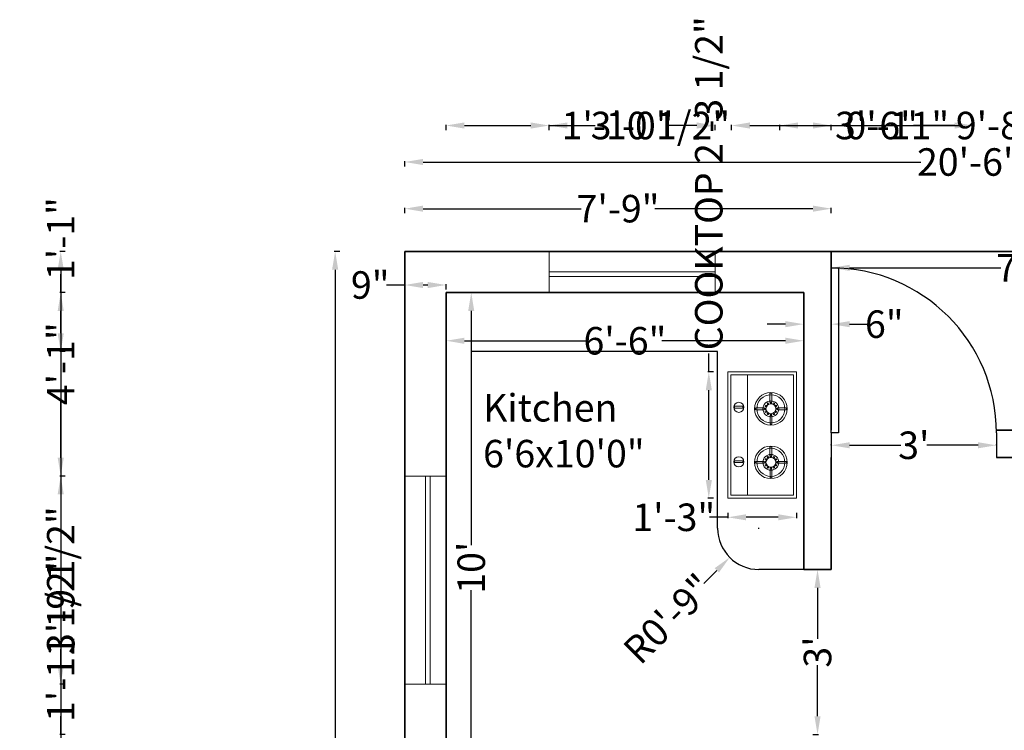
# Model space of a CAD drawing. Units: inches. Extents: x -81 to 380, y -521 to 79.
# Tile 3 of 5: x -81 to 134, y -76 to 79. Entities that reach past the tile are written whole.
import ezdxf

# ---------------------------------------------------------------- set-up
doc = ezdxf.new("R2010")
doc.units = ezdxf.units.IN
doc.header["$MEASUREMENT"] = 0
for name, color, linetype, lineweight in [('A-ANNO-DIMS', 2, 'Continuous', 18), ('A-AREA-IDEN', 5, 'Continuous', 25), ('A-EQPM', 8, 'Continuous', 18), ('A-FLOR-CASE', 249, 'Continuous', 25), ('A-GLAZ', 4, 'Continuous', 18), ('A-WALL', 249, 'Continuous', 35), ('door', 34, 'Continuous', 25)]:
    doc.layers.add(name, color=color, linetype=linetype, lineweight=lineweight)
doc.styles.get("Standard").update_dxf_attribs({"font": 'arial.ttf'})
doc.dimstyles.get("Standard").update_dxf_attribs({"dimtxt": 6, "dimasz": 4, "dimexe": 0.18, "dimexo": 0.0625, "dimgap": 0.09, "dimtad": 0, "dimdec": 0, "dimzin": 0, "dimdsep": 46, "dimlunit": 3, "dimtxsty": 'Standard', "dimcen": 0.09, "dimclrd": 6, "dimclre": 6, "dimclrt": 2, "dimadec": 0, "dimazin": 0, "dimtfac": 1, "dimtdec": 0, "dimtofl": 0, "dimtmove": 0, "dimatfit": 3, "dimfxl": 1, "dimfxlon": 1, "dimtolj": 1, "dimtzin": 0, "dimarcsym": 0})

# ---------------------------------------------------------------- blocks, each defined once
blk = doc.blocks.new('*U2')
for p, q in [((0, 0), (0, -6)), ((40, 0), (40, -6))]:
    blk.add_line(p, q)
blk.add_lwpolyline([(0, 0), (0, 40), (1.75, 40), (1.75, 0)], close=True)
blk.add_arc((0, 0), 40, 0, 90)
blk = doc.blocks.new('*D5')
at = {"layer": 'A-ANNO-DIMS', "color": 0, "lineweight": -2, "transparency": 16777216}
for p, q in [((3.31, 46.97), (3.31, 48.15)), ((7.31, 47.97), (115.86, 47.97)), ((245.31, 47.97), (136.76, 47.97)), ((249.31, 46.97), (249.31, 48.15))]:
    blk.add_line(p, q, dxfattribs=at)
at = {"layer": 'A-ANNO-DIMS', "color": 0, "transparency": 16777216}
for points in [[(7.31, 48.64), (7.31, 47.3), (3.31, 47.97)], [(245.31, 48.64), (245.31, 47.3), (249.31, 47.97)]]:
    blk.add_solid(points, dxfattribs=at)
at = {"layer": 'Defpoints', "color": 0, "transparency": 16777216}
for p in [(249.31, 47.97), (3.31, 28.48), (249.31, 28.48)]:
    blk.add_point(p, dxfattribs=at)
at = {"layer": 'A-ANNO-DIMS', "color": 0, "transparency": 16777216, "insert": (126.31, 47.97), "char_height": 6, "attachment_point": 5}
blk.add_mtext('\\A1;20\'-6"', dxfattribs=at)
blk = doc.blocks.new('*D6')
at = {"layer": 'A-ANNO-DIMS', "color": 0, "lineweight": -2, "transparency": 16777216}
for p, q in [((3.31, 21.14), (-0.69, 21.14)), ((3.31, 20.14), (3.31, 21.32)), ((8.31, 21.14), (7.31, 21.14)), ((12.31, 20.14), (12.31, 21.32))]:
    blk.add_line(p, q, dxfattribs=at)
at = {"layer": 'A-ANNO-DIMS', "color": 0, "transparency": 16777216}
for points in [[(7.31, 21.81), (7.31, 20.47), (3.31, 21.14)], [(8.31, 21.81), (8.31, 20.47), (12.31, 21.14)]]:
    blk.add_solid(points, dxfattribs=at)
at = {"layer": 'Defpoints', "color": 0, "transparency": 16777216}
for p in [(3.31, 21.14), (3.31, 19.48), (12.31, 19.48)]:
    blk.add_point(p, dxfattribs=at)
at = {"layer": 'A-ANNO-DIMS', "color": 0, "transparency": 16777216, "insert": (-4.23, 21.14), "char_height": 6, "attachment_point": 5}
blk.add_mtext('\\A1;9"', dxfattribs=at)
blk = doc.blocks.new('*D7')
at = {"layer": 'A-ANNO-DIMS', "color": 0, "lineweight": -2, "transparency": 16777216}
for p, q in [((90.31, 12.9), (90.31, 12.42)), ((96.31, 12.9), (96.31, 12.42)), ((86.31, 12.6), (82.31, 12.6)), ((100.31, 12.6), (104.31, 12.6))]:
    blk.add_line(p, q, dxfattribs=at)
at = {"layer": 'A-ANNO-DIMS', "color": 0, "transparency": 16777216}
for points in [[(86.31, 13.26), (86.31, 11.93), (90.31, 12.6)], [(100.31, 13.26), (100.31, 11.93), (96.31, 12.6)]]:
    blk.add_solid(points, dxfattribs=at)
at = {"layer": 'Defpoints', "color": 0, "transparency": 16777216}
for p in [(90.31, 12.96), (96.31, 12.96), (96.31, 12.6)]:
    blk.add_point(p, dxfattribs=at)
at = {"layer": 'A-ANNO-DIMS', "color": 0, "transparency": 16777216, "insert": (107.87, 12.6), "char_height": 6, "attachment_point": 5}
blk.add_mtext('\\A1;6"', dxfattribs=at)
blk = doc.blocks.new('*D8')
at = {"layer": 'A-ANNO-DIMS', "color": 0, "lineweight": -2, "transparency": 16777216}
for p, q in [((-10.88, 28.48), (-12.06, 28.48)), ((-11.88, 24.48), (-11.88, -110.29)), ((-11.88, -255.52), (-11.88, -120.75)), ((-10.88, -259.52), (-12.06, -259.52))]:
    blk.add_line(p, q, dxfattribs=at)
at = {"layer": 'A-ANNO-DIMS', "color": 0, "transparency": 16777216}
for points in [[(-12.55, 24.48), (-11.21, 24.48), (-11.88, 28.48)], [(-12.55, -255.52), (-11.21, -255.52), (-11.88, -259.52)]]:
    blk.add_solid(points, dxfattribs=at)
at = {"layer": 'Defpoints', "color": 0, "transparency": 16777216}
for p in [(3.31, 28.48), (-11.88, -259.52), (3.31, -259.52)]:
    blk.add_point(p, dxfattribs=at)
at = {"layer": 'A-ANNO-DIMS', "color": 0, "transparency": 16777216, "insert": (-11.88, -115.52), "char_height": 6, "attachment_point": 5, "rotation": 90}
blk.add_mtext("\\A1;24'", dxfattribs=at)
blk = doc.blocks.new('*D12')
at = {"layer": 'A-ANNO-DIMS', "color": 0, "lineweight": -2, "transparency": 16777216}
for p, q in [((3.31, 36.79), (3.31, 37.97)), ((7.31, 37.79), (41.77, 37.79)), ((92.31, 37.79), (57.85, 37.79)), ((96.31, 36.79), (96.31, 37.97))]:
    blk.add_line(p, q, dxfattribs=at)
at = {"layer": 'A-ANNO-DIMS', "color": 0, "transparency": 16777216}
for points in [[(7.31, 38.46), (7.31, 37.12), (3.31, 37.79)], [(92.31, 38.46), (92.31, 37.12), (96.31, 37.79)]]:
    blk.add_solid(points, dxfattribs=at)
at = {"layer": 'Defpoints', "color": 0, "transparency": 16777216}
for p in [(96.31, 37.79), (3.31, 28.48), (96.31, 28.48)]:
    blk.add_point(p, dxfattribs=at)
at = {"layer": 'A-ANNO-DIMS', "color": 0, "transparency": 16777216, "insert": (49.81, 37.79), "char_height": 6, "attachment_point": 5}
blk.add_mtext('\\A1;7\'-9"', dxfattribs=at)
blk = doc.blocks.new('*D13')
at = {"layer": 'A-ANNO-DIMS', "color": 0, "lineweight": -2, "transparency": 16777216}
for p, q in [((18.8, 19.48), (17.62, 19.48)), ((17.8, 15.48), (17.8, -35.62)), ((17.8, -96.52), (17.8, -45.42)), ((18.8, -100.52), (17.62, -100.52))]:
    blk.add_line(p, q, dxfattribs=at)
at = {"layer": 'A-ANNO-DIMS', "color": 0, "transparency": 16777216}
for points in [[(17.13, 15.48), (18.46, 15.48), (17.8, 19.48)], [(17.13, -96.52), (18.46, -96.52), (17.8, -100.52)]]:
    blk.add_solid(points, dxfattribs=at)
at = {"layer": 'Defpoints', "color": 0, "transparency": 16777216}
for p in [(17.8, 19.48), (28.81, 19.48), (28.81, -100.52)]:
    blk.add_point(p, dxfattribs=at)
at = {"layer": 'A-ANNO-DIMS', "color": 0, "transparency": 16777216, "insert": (17.8, -40.52), "char_height": 6, "attachment_point": 5, "rotation": 90}
blk.add_mtext("\\A1;10'", dxfattribs=at)
blk = doc.blocks.new('*D14')
at = {"layer": 'A-ANNO-DIMS', "color": 0, "lineweight": -2, "transparency": 16777216}
for p, q in [((12.31, 8.08), (12.31, 9.16)), ((16.31, 8.98), (43.23, 8.98)), ((86.31, 8.98), (59.39, 8.98)), ((90.31, 8.98), (90.31, 9.16))]:
    blk.add_line(p, q, dxfattribs=at)
at = {"layer": 'A-ANNO-DIMS', "color": 0, "transparency": 16777216}
for points in [[(16.31, 9.65), (16.31, 8.31), (12.31, 8.98)], [(86.31, 9.65), (86.31, 8.31), (90.31, 8.98)]]:
    blk.add_solid(points, dxfattribs=at)
at = {"layer": 'Defpoints', "color": 0, "transparency": 16777216}
for p in [(90.31, 8.98), (90.31, 8.98), (12.31, 8.01)]:
    blk.add_point(p, dxfattribs=at)
at = {"layer": 'A-ANNO-DIMS', "color": 0, "transparency": 16777216, "insert": (51.31, 8.98), "char_height": 6, "attachment_point": 5}
blk.add_mtext('\\A1;6\'-6"', dxfattribs=at)
blk = doc.blocks.new('*D15')
at = {"layer": 'A-ANNO-DIMS', "color": 0, "lineweight": -2, "transparency": 16777216}
for p, q in [((96.31, 24.88), (96.31, 25.06)), ((100.31, 24.88), (133.27, 24.88)), ((182.31, 24.88), (149.35, 24.88)), ((186.31, 24.88), (186.31, 25.06))]:
    blk.add_line(p, q, dxfattribs=at)
at = {"layer": 'A-ANNO-DIMS', "color": 0, "transparency": 16777216}
for points in [[(100.31, 25.55), (100.31, 24.21), (96.31, 24.88)], [(182.31, 25.55), (182.31, 24.21), (186.31, 24.88)]]:
    blk.add_solid(points, dxfattribs=at)
at = {"layer": 'Defpoints', "color": 0, "transparency": 16777216}
for p in [(96.31, 24.88), (186.31, 24.88), (186.31, 24.88)]:
    blk.add_point(p, dxfattribs=at)
at = {"layer": 'A-ANNO-DIMS', "color": 0, "transparency": 16777216, "insert": (141.31, 24.88), "char_height": 6, "attachment_point": 5}
blk.add_mtext('\\A1;7\'-6"', dxfattribs=at)
blk = doc.blocks.new('*D27')
at = {"layer": 'A-ANNO-DIMS', "color": 0, "lineweight": -2, "transparency": 16777216}
for p, q in [((96.31, -13.82), (96.31, -13.64)), ((100.31, -13.82), (111.46, -13.82)), ((128.31, -13.82), (117.16, -13.82)), ((132.31, -13.82), (132.31, -13.64))]:
    blk.add_line(p, q, dxfattribs=at)
at = {"layer": 'A-ANNO-DIMS', "color": 0, "transparency": 16777216}
for points in [[(100.31, -13.15), (100.31, -14.49), (96.31, -13.82)], [(128.31, -13.15), (128.31, -14.49), (132.31, -13.82)]]:
    blk.add_solid(points, dxfattribs=at)
at = {"layer": 'Defpoints', "color": 0, "transparency": 16777216}
for p in [(96.31, -13.82), (132.31, -13.82), (132.31, -13.82)]:
    blk.add_point(p, dxfattribs=at)
at = {"layer": 'A-ANNO-DIMS', "color": 0, "transparency": 16777216, "insert": (114.31, -13.82), "char_height": 6, "attachment_point": 5}
blk.add_mtext("\\A1;3'", dxfattribs=at)
blk = doc.blocks.new('*D28')
at = {"layer": 'A-ANNO-DIMS', "color": 0, "lineweight": -2, "transparency": 16777216}
for p, q in [((92.31, -40.92), (93.49, -40.92)), ((93.31, -44.92), (93.31, -56.07)), ((93.31, -72.92), (93.31, -61.76)), ((92.31, -76.92), (93.49, -76.92))]:
    blk.add_line(p, q, dxfattribs=at)
at = {"layer": 'A-ANNO-DIMS', "color": 0, "transparency": 16777216}
for points in [[(92.64, -44.92), (93.98, -44.92), (93.31, -40.92)], [(92.64, -72.92), (93.98, -72.92), (93.31, -76.92)]]:
    blk.add_solid(points, dxfattribs=at)
at = {"layer": 'Defpoints', "color": 0, "transparency": 16777216}
for p in [(90.31, -40.92), (93.31, -40.92), (90.31, -76.92)]:
    blk.add_point(p, dxfattribs=at)
at = {"layer": 'A-ANNO-DIMS', "color": 0, "transparency": 16777216, "insert": (93.31, -58.92), "char_height": 6, "attachment_point": 5, "rotation": 90}
blk.add_mtext("\\A1;3'", dxfattribs=at)
blk = doc.blocks.new('A$C06E242FC')
for p, q in [((0, 455.6), (0.5, 456.1)), ((0, 455.6), (0, 0.5)), ((838.9, 456.1), (0.5, 456.1)), ((20, 435.6), (20.5, 436.1)), ((20, 435.6), (20, 20.5)), ((818.9, 436.1), (20.5, 436.1)), ((237.3, 411.5), (237.3, 356.2)), ((248.9, 411.5), (237.3, 411.5)), ((248.9, 356.2), (248.9, 411.5)), ((599.3, 411.5), (610.9, 411.5)), ((599.3, 411.5), (599.3, 356.2)), ((610.9, 356.2), (610.9, 411.5)), ((819.4, 435.6), (818.9, 436.1)), ((819.4, 20.5), (819.4, 435.6)), ((838.9, 456.1), (839.4, 455.6)), ((839.4, 0.5), (839.4, 455.6)), ((237.3, 356.2), (248.9, 356.2)), ((599.3, 356.2), (610.9, 356.2)), ((20, 324.4), (819.4, 324.4)), ((232.7, 272.7), (232.7, 214)), ((244.9, 272.7), (232.7, 272.7)), ((244.9, 214), (244.9, 272.7)), ((588.1, 272.7), (588.1, 214)), ((600.3, 272.7), (588.1, 272.7)), ((600.3, 214), (600.3, 272.7)), ((232.7, 214), (244.9, 214)), ((588.1, 214), (600.3, 214)), ((136.3, 176), (136.3, 163.8)), ((194.9, 176), (136.3, 176)), ((136.3, 163.8), (194.9, 163.8)), ((194.9, 163.8), (194.9, 176)), ((282.9, 176.3), (282.9, 164.1)), ((341.6, 176.3), (282.9, 176.3)), ((282.9, 164.1), (341.6, 164.1)), ((341.6, 164.1), (341.6, 176.3)), ((550.3, 176), (491.7, 176)), ((491.7, 176), (491.7, 163.8)), ((491.7, 163.8), (550.3, 163.8)), ((550.3, 163.8), (550.3, 176)), ((638.3, 176.3), (638.3, 164.1)), ((697, 176.3), (638.3, 176.3)), ((638.3, 164.1), (697, 164.1)), ((697, 164.1), (697, 176.3)), ((245.2, 126.1), (233, 126.1)), ((233, 126.1), (233, 67.4)), ((233, 67.4), (245.2, 67.4)), ((245.2, 67.4), (245.2, 126.1)), ((600.6, 126.1), (588.3, 126.1)), ((588.3, 126.1), (588.3, 67.4)), ((588.3, 67.4), (600.6, 67.4)), ((600.6, 67.4), (600.6, 126.1)), ((0, 0.5), (0.5, 0)), ((20, 20.5), (20.5, 20)), ((20.5, 20), (818.9, 20)), ((818.9, 20), (819.4, 20.5)), ((838.9, 0), (839.4, 0.5)), ((0.5, 0), (838.9, 0))]:
    blk.add_line(p, q)
for centre, radius in [((242, 382.9), 33.3), ((604.1, 382.9), 33.3), ((238.9, 170.1), 108.3), ((238.9, 170.1), 93.3), ((594.3, 170.1), 108.3), ((594.3, 170.1), 93.3), ((238.9, 170.1), 52.6), ((238.9, 170.1), 32.6), ((219.5, 203.7), 4.84), ((238.9, 208.9), 4.84), ((258.4, 203.7), 4.84), ((594.3, 170.1), 52.6), ((594.3, 170.1), 32.6), ((574.9, 203.7), 4.84), ((594.3, 208.9), 4.84), ((613.7, 203.7), 4.84), ((200.1, 170.1), 4.84), ((205.3, 189.5), 4.84), ((205.3, 150.6), 4.84), ((219.5, 136.4), 4.84), ((238.9, 131.2), 4.84), ((258.4, 136.4), 4.84), ((272.6, 189.5), 4.84), ((272.6, 150.6), 4.84), ((277.8, 170.1), 4.84), ((555.5, 170.1), 4.84), ((560.7, 189.5), 4.84), ((560.7, 150.6), 4.84), ((574.9, 136.4), 4.84), ((594.3, 131.2), 4.84), ((613.7, 136.4), 4.84), ((628, 189.5), 4.84), ((628, 150.6), 4.84), ((633.2, 170.1), 4.84)]:
    blk.add_circle(centre, radius)
blk = doc.blocks.new('*D44')
at = {"layer": 'A-ANNO-DIMS', "color": 6, "lineweight": -2, "transparency": 16777216}
for p, q in [((69.6, 2.19), (69.6, 6.19)), ((70.6, 2.19), (69.42, 2.19)), ((69.6, -21.39), (69.6, -1.81)), ((70.6, -25.39), (69.42, -25.39))]:
    blk.add_line(p, q, dxfattribs=at)
at = {"layer": 'A-ANNO-DIMS', "color": 6, "transparency": 16777216}
for points in [[(68.94, -1.81), (70.27, -1.81), (69.6, 2.19)], [(68.94, -21.39), (70.27, -21.39), (69.6, -25.39)]]:
    blk.add_solid(points, dxfattribs=at)
at = {"layer": 'Defpoints', "color": 0, "transparency": 16777216}
for p in [(69.6, 2.19), (73.74, 2.19), (73.74, -25.39)]:
    blk.add_point(p, dxfattribs=at)
at = {"layer": 'A-ANNO-DIMS', "color": 2, "transparency": 16777216, "insert": (69.6, 43.33), "char_height": 6, "attachment_point": 5, "rotation": 90}
blk.add_mtext('\\A1;COOKTOP 2\'-3 1/2"', dxfattribs=at)
blk = doc.blocks.new('*D45')
at = {"layer": 'A-ANNO-DIMS', "color": 6, "lineweight": -2, "transparency": 16777216}
for p, q in [((73.74, -29.53), (69.74, -29.53)), ((73.74, -28.53), (73.74, -29.71)), ((84.73, -29.53), (77.74, -29.53)), ((88.73, -28.53), (88.73, -29.71))]:
    blk.add_line(p, q, dxfattribs=at)
at = {"layer": 'A-ANNO-DIMS', "color": 6, "transparency": 16777216}
for points in [[(77.74, -28.86), (77.74, -30.2), (73.74, -29.53)], [(84.73, -28.86), (84.73, -30.2), (88.73, -29.53)]]:
    blk.add_solid(points, dxfattribs=at)
at = {"layer": 'Defpoints', "color": 0, "transparency": 16777216}
for p in [(73.74, -25.39), (88.73, -25.39), (73.74, -29.53)]:
    blk.add_point(p, dxfattribs=at)
at = {"layer": 'A-ANNO-DIMS', "color": 2, "transparency": 16777216, "insert": (61.96, -29.53), "char_height": 6, "attachment_point": 5}
blk.add_mtext('\\A1;1\'-3"', dxfattribs=at)
blk = doc.blocks.new('*D46')
at = {"layer": 'A-ANNO-DIMS', "color": 6, "lineweight": -2, "transparency": 16777216}
for p, q in [((74.55, 54.93), (74.55, 56.11)), ((78.55, 55.93), (124.45, 55.93)), ((186.48, 55.93), (140.58, 55.93)), ((190.48, 54.93), (190.48, 56.11))]:
    blk.add_line(p, q, dxfattribs=at)
at = {"layer": 'A-ANNO-DIMS', "color": 6, "transparency": 16777216}
for points in [[(78.55, 56.6), (78.55, 55.26), (74.55, 55.93)], [(186.48, 56.6), (186.48, 55.26), (190.48, 55.93)]]:
    blk.add_solid(points, dxfattribs=at)
at = {"layer": 'Defpoints', "color": 0, "transparency": 16777216}
for p in [(190.48, 55.93), (74.55, -489.67), (190.48, -489.67)]:
    blk.add_point(p, dxfattribs=at)
at = {"layer": 'A-ANNO-DIMS', "color": 2, "transparency": 16777216, "insert": (132.51, 55.93), "char_height": 6, "attachment_point": 5}
blk.add_mtext('\\A1;9\'-8"', dxfattribs=at)
blk = doc.blocks.new('*D48')
at = {"layer": 'A-ANNO-DIMS', "color": 6, "lineweight": -2, "transparency": 16777216}
for p, q in [((-70.72, 28.48), (-71.9, 28.48)), ((-71.72, 24.48), (-71.72, -220.08)), ((-71.72, -485.67), (-71.72, -241.11)), ((-70.72, -489.67), (-71.9, -489.67))]:
    blk.add_line(p, q, dxfattribs=at)
at = {"layer": 'A-ANNO-DIMS', "color": 6, "transparency": 16777216}
for points in [[(-72.39, 24.48), (-71.06, 24.48), (-71.72, 28.48)], [(-72.39, -485.67), (-71.06, -485.67), (-71.72, -489.67)]]:
    blk.add_solid(points, dxfattribs=at)
at = {"layer": 'Defpoints', "color": 0, "transparency": 16777216}
for p in [(3.31, 28.48), (-71.72, -489.67), (74.55, -489.67)]:
    blk.add_point(p, dxfattribs=at)
at = {"layer": 'A-ANNO-DIMS', "color": 2, "transparency": 16777216, "insert": (-71.72, -230.6), "char_height": 6, "attachment_point": 5, "rotation": 90}
blk.add_mtext('\\A1;43\'-2"', dxfattribs=at)
blk = doc.blocks.new('*D50')
at = {"layer": 'A-ANNO-DIMS', "color": 6, "lineweight": -2, "transparency": 16777216}
for p, q in [((85.08, 54.93), (85.08, 56.11)), ((89.08, 55.93), (98.09, 55.93)), ((123.23, 55.93), (114.22, 55.93)), ((127.23, 54.93), (127.23, 56.11))]:
    blk.add_line(p, q, dxfattribs=at)
at = {"layer": 'A-ANNO-DIMS', "color": 6, "transparency": 16777216}
for points in [[(89.08, 56.6), (89.08, 55.26), (85.08, 55.93)], [(123.23, 56.6), (123.23, 55.26), (127.23, 55.93)]]:
    blk.add_solid(points, dxfattribs=at)
at = {"layer": 'Defpoints', "color": 0, "transparency": 16777216}
for p in [(127.23, 55.93), (85.08, -292.11), (127.23, -292.11)]:
    blk.add_point(p, dxfattribs=at)
at = {"layer": 'A-ANNO-DIMS', "color": 2, "transparency": 16777216, "insert": (106.16, 55.93), "char_height": 6, "attachment_point": 5}
blk.add_mtext('\\A1;3\'-6"', dxfattribs=at)
blk = doc.blocks.new('*D53')
at = {"layer": 'A-ANNO-DIMS', "color": 6, "lineweight": -2, "transparency": 16777216}
for p, q in [((85.08, 54.93), (85.08, 56.11)), ((89.08, 55.93), (92.31, 55.93)), ((96.31, 54.93), (96.31, 56.11)), ((96.31, 55.93), (100.31, 55.93))]:
    blk.add_line(p, q, dxfattribs=at)
at = {"layer": 'A-ANNO-DIMS', "color": 6, "transparency": 16777216}
for points in [[(89.08, 56.6), (89.08, 55.26), (85.08, 55.93)], [(92.31, 56.6), (92.31, 55.26), (96.31, 55.93)]]:
    blk.add_solid(points, dxfattribs=at)
at = {"layer": 'Defpoints', "color": 0, "transparency": 16777216}
for p in [(96.31, 55.93), (85.08, -259.52), (96.31, -259.52)]:
    blk.add_point(p, dxfattribs=at)
at = {"layer": 'A-ANNO-DIMS', "color": 2, "transparency": 16777216, "insert": (110.71, 55.93), "char_height": 6, "attachment_point": 5}
blk.add_mtext('\\A1;0\'-11"', dxfattribs=at)
blk = doc.blocks.new('*D54')
at = {"layer": 'A-ANNO-DIMS', "color": 6, "lineweight": -2, "transparency": 16777216}
for p, q in [((370.52, 19.48), (371.7, 19.48)), ((371.52, 15.48), (371.52, 4.34)), ((371.52, -36.92), (371.52, -25.77)), ((370.52, -40.92), (371.7, -40.92))]:
    blk.add_line(p, q, dxfattribs=at)
at = {"layer": 'A-ANNO-DIMS', "color": 6, "transparency": 16777216}
for points in [[(370.86, 15.48), (372.19, 15.48), (371.52, 19.48)], [(370.86, -36.92), (372.19, -36.92), (371.52, -40.92)]]:
    blk.add_solid(points, dxfattribs=at)
at = {"layer": 'Defpoints', "color": 0, "transparency": 16777216}
for p in [(90.31, 19.48), (90.31, -40.92), (371.52, -40.92)]:
    blk.add_point(p, dxfattribs=at)
at = {"layer": 'A-ANNO-DIMS', "color": 2, "transparency": 16777216, "insert": (371.52, -10.72), "char_height": 6, "attachment_point": 5, "rotation": 90}
blk.add_mtext('\\A1;5\'-0 1/2"', dxfattribs=at)
blk = doc.blocks.new('*D55')
at = {"layer": 'A-ANNO-DIMS', "color": 6, "lineweight": -2, "transparency": 16777216}
for p, q in [((67.53, -517.12), (63.53, -517.12)), ((71.53, -516.12), (71.53, -517.3)), ((90.31, -516.12), (90.31, -517.3)), ((94.31, -517.12), (98.31, -517.12))]:
    blk.add_line(p, q, dxfattribs=at)
at = {"layer": 'A-ANNO-DIMS', "color": 6, "transparency": 16777216}
for points in [[(67.53, -516.45), (67.53, -517.79), (71.53, -517.12)], [(94.31, -516.45), (94.31, -517.79), (90.31, -517.12)]]:
    blk.add_solid(points, dxfattribs=at)
at = {"layer": 'Defpoints', "color": 0, "transparency": 16777216}
for p in [(71.53, -31.92), (90.31, -40.92), (90.31, -517.12)]:
    blk.add_point(p, dxfattribs=at)
at = {"layer": 'A-ANNO-DIMS', "color": 2, "transparency": 16777216, "insert": (80.92, -517.12), "char_height": 6, "attachment_point": 5}
blk.add_mtext('\\A1;1\'-7"', dxfattribs=at)
blk = doc.blocks.new('*D56')
at = {"layer": 'A-ANNO-DIMS', "color": 6, "lineweight": -2, "transparency": 16777216}
for p, q in [((-71.72, 19.48), (-71.72, 23.48)), ((-70.72, 19.48), (-71.9, 19.48)), ((-71.72, 10.6), (-71.72, 15.48)), ((-70.72, 6.6), (-71.9, 6.6))]:
    blk.add_line(p, q, dxfattribs=at)
at = {"layer": 'A-ANNO-DIMS', "color": 6, "transparency": 16777216}
for points in [[(-72.39, 15.48), (-71.06, 15.48), (-71.72, 19.48)], [(-72.39, 10.6), (-71.06, 10.6), (-71.72, 6.6)]]:
    blk.add_solid(points, dxfattribs=at)
at = {"layer": 'Defpoints', "color": 0, "transparency": 16777216}
for p in [(-71.72, 19.48), (12.31, 19.48), (17.8, 6.6)]:
    blk.add_point(p, dxfattribs=at)
at = {"layer": 'A-ANNO-DIMS', "color": 2, "transparency": 16777216, "insert": (-71.72, 31.26), "char_height": 6, "attachment_point": 5, "rotation": 90}
blk.add_mtext('\\A1;1\'-1"', dxfattribs=at)
blk = doc.blocks.new('*D57')
at = {"layer": 'A-ANNO-DIMS', "color": 6, "lineweight": -2, "transparency": 16777216}
for p, q in [((-71.72, -76.92), (-71.72, -72.92)), ((-70.72, -76.92), (-71.9, -76.92)), ((-71.72, -96.52), (-71.72, -80.92)), ((-70.72, -100.52), (-71.9, -100.52))]:
    blk.add_line(p, q, dxfattribs=at)
at = {"layer": 'A-ANNO-DIMS', "color": 6, "transparency": 16777216}
for points in [[(-72.39, -80.92), (-71.06, -80.92), (-71.72, -76.92)], [(-72.39, -96.52), (-71.06, -96.52), (-71.72, -100.52)]]:
    blk.add_solid(points, dxfattribs=at)
at = {"layer": 'Defpoints', "color": 0, "transparency": 16777216}
for p in [(-71.72, -76.92), (45.3, -76.92), (45.3, -100.52)]:
    blk.add_point(p, dxfattribs=at)
at = {"layer": 'A-ANNO-DIMS', "color": 2, "transparency": 16777216, "insert": (-71.72, -55.81), "char_height": 6, "attachment_point": 5, "rotation": 90}
blk.add_mtext('\\A1;1\'-11 1/2"', dxfattribs=at)
blk = doc.blocks.new('*D59')
at = {"layer": 'A-ANNO-DIMS', "color": 6, "lineweight": -2, "transparency": 16777216}
for p, q in [((370.52, -25.38), (371.7, -25.38)), ((371.52, -29.38), (371.52, -36.92)), ((370.52, -40.92), (371.7, -40.92)), ((371.52, -40.92), (371.52, -44.92))]:
    blk.add_line(p, q, dxfattribs=at)
at = {"layer": 'A-ANNO-DIMS', "color": 6, "transparency": 16777216}
for points in [[(370.86, -29.38), (372.19, -29.38), (371.52, -25.38)], [(370.86, -36.92), (372.19, -36.92), (371.52, -40.92)]]:
    blk.add_solid(points, dxfattribs=at)
at = {"layer": 'Defpoints', "color": 0, "transparency": 16777216}
for p in [(88.73, -25.38), (90.31, -40.92), (371.52, -40.92)]:
    blk.add_point(p, dxfattribs=at)
at = {"layer": 'A-ANNO-DIMS', "color": 2, "transparency": 16777216, "insert": (371.52, -59.69), "char_height": 6, "attachment_point": 5, "rotation": 90}
blk.add_mtext('\\A1;1\'-3 1/2"', dxfattribs=at)
blk = doc.blocks.new('*D60')
at = {"layer": 'A-ANNO-DIMS', "color": 6, "lineweight": -2, "transparency": 16777216}
for p, q in [((34.77, 54.93), (34.77, 56.11)), ((38.77, 55.93), (44.82, 55.93)), ((66.99, 55.93), (60.94, 55.93)), ((70.99, 54.93), (70.99, 56.11))]:
    blk.add_line(p, q, dxfattribs=at)
at = {"layer": 'A-ANNO-DIMS', "color": 6, "transparency": 16777216}
for points in [[(38.77, 56.6), (38.77, 55.26), (34.77, 55.93)], [(66.99, 56.6), (66.99, 55.26), (70.99, 55.93)]]:
    blk.add_solid(points, dxfattribs=at)
at = {"layer": 'Defpoints', "color": 0, "transparency": 16777216}
for p in [(70.99, 55.93), (34.77, 28.48), (70.99, 28.48)]:
    blk.add_point(p, dxfattribs=at)
at = {"layer": 'A-ANNO-DIMS', "color": 2, "transparency": 16777216, "insert": (52.88, 55.93), "char_height": 6, "attachment_point": 5}
blk.add_mtext('\\A1;3\'-0"', dxfattribs=at)
blk = doc.blocks.new('*D61')
at = {"layer": 'A-ANNO-DIMS', "color": 6, "lineweight": -2, "transparency": 16777216}
for p, q in [((-70.72, -20.53), (-71.9, -20.53)), ((-71.72, -24.53), (-71.72, -28.19)), ((-71.72, -61.95), (-71.72, -58.29)), ((-70.72, -65.95), (-71.9, -65.95))]:
    blk.add_line(p, q, dxfattribs=at)
at = {"layer": 'A-ANNO-DIMS', "color": 6, "transparency": 16777216}
for points in [[(-72.39, -24.53), (-71.06, -24.53), (-71.72, -20.53)], [(-72.39, -61.95), (-71.06, -61.95), (-71.72, -65.95)]]:
    blk.add_solid(points, dxfattribs=at)
at = {"layer": 'Defpoints', "color": 0, "transparency": 16777216}
for p in [(3.31, -20.53), (-71.72, -65.95), (3.31, -65.95)]:
    blk.add_point(p, dxfattribs=at)
at = {"layer": 'A-ANNO-DIMS', "color": 2, "transparency": 16777216, "insert": (-71.72, -43.24), "char_height": 6, "attachment_point": 5, "rotation": 90}
blk.add_mtext('\\A1;3\'-9 1/2"', dxfattribs=at)
blk = doc.blocks.new('*D62')
at = {"layer": 'A-ANNO-DIMS', "color": 6, "lineweight": -2, "transparency": 16777216}
for p, q in [((12.31, 54.93), (12.31, 56.11)), ((16.31, 55.93), (30.77, 55.93)), ((34.77, 54.93), (34.77, 56.11)), ((34.77, 55.93), (38.77, 55.93))]:
    blk.add_line(p, q, dxfattribs=at)
at = {"layer": 'A-ANNO-DIMS', "color": 6, "transparency": 16777216}
for points in [[(16.31, 56.6), (16.31, 55.26), (12.31, 55.93)], [(30.77, 56.6), (30.77, 55.26), (34.77, 55.93)]]:
    blk.add_solid(points, dxfattribs=at)
at = {"layer": 'Defpoints', "color": 0, "transparency": 16777216}
for p in [(34.77, 55.93), (12.31, 19.48), (34.77, 19.48)]:
    blk.add_point(p, dxfattribs=at)
at = {"layer": 'A-ANNO-DIMS', "color": 2, "transparency": 16777216, "insert": (55.88, 55.93), "char_height": 6, "attachment_point": 5}
blk.add_mtext('\\A1;1\'-10 1/2"', dxfattribs=at)
blk = doc.blocks.new('*D63')
at = {"layer": 'A-ANNO-DIMS', "color": 6, "lineweight": -2, "transparency": 16777216}
for p, q in [((-70.72, 28.48), (-71.9, 28.48)), ((-71.72, 24.48), (-71.72, 12.16)), ((-71.72, -16.53), (-71.72, -4.21)), ((-70.72, -20.53), (-71.9, -20.53))]:
    blk.add_line(p, q, dxfattribs=at)
at = {"layer": 'A-ANNO-DIMS', "color": 6, "transparency": 16777216}
for points in [[(-72.39, 24.48), (-71.06, 24.48), (-71.72, 28.48)], [(-72.39, -16.53), (-71.06, -16.53), (-71.72, -20.53)]]:
    blk.add_solid(points, dxfattribs=at)
at = {"layer": 'Defpoints', "color": 0, "transparency": 16777216}
for p in [(3.31, 28.48), (-71.72, -20.53), (3.31, -20.53)]:
    blk.add_point(p, dxfattribs=at)
at = {"layer": 'A-ANNO-DIMS', "color": 2, "transparency": 16777216, "insert": (-71.72, 3.97), "char_height": 6, "attachment_point": 5, "rotation": 90}
blk.add_mtext('\\A1;4\'-1"', dxfattribs=at)
blk = doc.blocks.new('*D69')
at = {"layer": 'A-ANNO-DIMS', "color": 6, "lineweight": -2, "transparency": 16777216}
for p, q in [((80.44, -31.92), (80.62, -31.92)), ((80.53, -32.01), (80.53, -31.83)), ((68.51, -43.94), (71.33, -41.11))]:
    blk.add_line(p, q, dxfattribs=at)
at = {"layer": 'A-ANNO-DIMS', "color": 6, "transparency": 16777216}
blk.add_solid([(70.86, -40.64), (71.81, -41.58), (74.16, -38.28)], dxfattribs=at)
at = {"layer": 'Defpoints', "color": 0, "transparency": 16777216}
for p in [(80.53, -31.92), (74.16, -38.28)]:
    blk.add_point(p, dxfattribs=at)
at = {"layer": 'A-ANNO-DIMS', "color": 2, "transparency": 16777216, "insert": (60.77, -51.67), "char_height": 6, "attachment_point": 5, "rotation": 44.9996}
blk.add_mtext('\\A1;R0\'-9"', dxfattribs=at)

msp = doc.modelspace()

# ---------------------------------------------------------------- linework, layer by layer
at = {"layer": 'A-FLOR-CASE'}
for p, q in [((71.53, 6.6), (17.8, 6.6)), ((71.53, -31.92), (71.53, 6.6)), ((90.31, -40.92), (80.53, -40.92))]:
    msp.add_line(p, q, dxfattribs=at)
msp.add_arc((80.53, -31.92), 9, 180, 270, dxfattribs=at)
at = {"layer": 'A-GLAZ'}
for p, q in [((34.77, 28.48), (34.77, 19.48)), ((70.99, 28.48), (70.99, 19.48)), ((70.99, 23.98), (34.77, 23.98)), ((70.99, 22.98), (34.77, 22.98)), ((12.31, -20.53), (3.31, -20.53)), ((7.81, -20.53), (7.81, -65.95)), ((8.81, -20.53), (8.81, -65.95)), ((12.31, -65.95), (3.31, -65.95))]:
    msp.add_line(p, q, dxfattribs=at)
at = {"layer": 'A-WALL'}
for p, q in [((3.31, 28.48), (249.31, 28.48)), ((3.31, 28.48), (3.31, -259.52)), ((96.31, 28.48), (96.31, -10.52)), ((12.31, 19.48), (90.31, 19.48)), ((12.31, 19.48), (12.31, -100.52)), ((90.31, 19.48), (90.31, -40.92)), ((132.31, -10.52), (186.31, -10.52)), ((96.31, -16.52), (96.31, -40.92)), ((132.31, -16.52), (186.31, -16.52)), ((90.31, -40.92), (96.31, -40.92))]:
    msp.add_line(p, q, dxfattribs=at)

# ---------------------------------------------------------------- block references
at = {"layer": 'A-EQPM', "xscale": 0.0328579488209242, "yscale": 0.0328579488209242, "zscale": 0.0328579488209242, "rotation": 89.99999999999999}
msp.add_blockref('A$C06E242FC', (88.73, -25.39), dxfattribs=at)
at = {"layer": 'door', "xscale": 0.9, "yscale": 0.9, "zscale": 0.9}
msp.add_blockref('*U2', (96.31, -11.12), dxfattribs=at)

# ---------------------------------------------------------------- texts
at = {"layer": 'A-AREA-IDEN', "insert": (20.38, -2.64), "char_height": 6, "attachment_point": 1}
msp.add_mtext_dynamic_manual_height_columns('Kitchen\\P6\'6x10\'0"', width=81.6384, gutter_width=1, heights=[0], dxfattribs=at)

# ---------------------------------------------------------------- dimensions: what is measured, and where the dimension line sits
at = {"layer": 'A-ANNO-DIMS'}
dim = msp.add_linear_dim(base=(69.6, 2.19), p1=(73.74, -25.39), p2=(73.74, 2.19), angle=90, text='COOKTOP <>', dimstyle='Standard', override={"dimdec": 1, "dimlfac": 1, "dimrnd": 0, "dimzin": 1, "dimdsep": 46, "dimlunit": 4, "dimfrac": 2}, dxfattribs=at)
dim.commit()
dim.dimension.update_dxf_attribs({"geometry": '*D44', "text_midpoint": (69.6, 43.33)})
for base, p1, p2, override, picture, middle in [((34.77, 55.93), (12.31, 19.48), (34.77, 19.48), {"dimdec": 1, "dimlfac": 1, "dimrnd": 0, "dimzin": 1, "dimdsep": 46, "dimlunit": 4, "dimfrac": 2}, '*D62', (55.88, 55.93)), ((70.99, 55.93), (34.77, 28.48), (70.99, 28.48), {"dimdec": 1, "dimlfac": 1, "dimrnd": 0, "dimzin": 1, "dimdsep": 46, "dimlunit": 4, "dimfrac": 2}, '*D60', (52.88, 55.93)), ((190.48, 55.93), (74.55, -489.67), (190.48, -489.67), {"dimdec": 1, "dimlfac": 1, "dimrnd": 0, "dimzin": 1, "dimdsep": 46, "dimlunit": 4, "dimfrac": 2}, '*D46', (132.51, 55.93)), ((127.2309, 55.9306), (85.0832, -292.1074), (127.2309, -292.1074), {"dimdec": 1, "dimlfac": 1, "dimrnd": 0, "dimzin": 1, "dimdsep": 46, "dimlunit": 4, "dimfrac": 2}, '*D50', (106.1571, 55.9306)), ((96.31, 55.93), (85.08, -259.52), (96.31, -259.52), {"dimdec": 1, "dimlfac": 1, "dimrnd": 0, "dimzin": 1, "dimdsep": 46, "dimlunit": 4, "dimfrac": 2}, '*D53', (110.71, 55.93)), ((249.31, 47.97), (3.31, 28.48), (249.31, 28.48), {"dimclrd": 0, "dimclre": 0, "dimclrt": 0}, '*D5', (126.31, 47.97)), ((96.31, 37.79), (3.31, 28.48), (96.31, 28.48), {"dimclrd": 0, "dimclre": 0, "dimclrt": 0}, '*D12', (49.81, 37.79)), ((186.31, 24.88), (96.31, 24.88), (186.31, 24.88), {"dimclrd": 0, "dimclre": 0, "dimclrt": 0}, '*D15', (141.31, 24.88)), ((3.31, 21.14), (12.31, 19.48), (3.31, 19.48), {"dimclrd": 0, "dimclre": 0, "dimclrt": 0}, '*D6', (-4.23, 21.14)), ((96.31, 12.6), (90.31, 12.96), (96.31, 12.96), {"dimclrd": 0, "dimclre": 0, "dimclrt": 0}, '*D7', (107.87, 12.6)), ((90.31, 8.98), (12.31, 8.01), (90.31, 8.98), {"dimclrd": 0, "dimclre": 0, "dimclrt": 0}, '*D14', (51.31, 8.98)), ((132.31, -13.82), (96.31, -13.82), (132.31, -13.82), {"dimclrd": 0, "dimclre": 0, "dimclrt": 0}, '*D27', (114.31, -13.82)), ((90.31, -517.12), (71.53, -31.92), (90.31, -40.92), {"dimdec": 1, "dimlfac": 1, "dimrnd": 0, "dimzin": 1, "dimdsep": 46, "dimlunit": 4, "dimfrac": 2}, '*D55', (80.92, -517.12))]:
    dim = msp.add_linear_dim(base=base, p1=p1, p2=p2, dimstyle='Standard', override=override, dxfattribs=at)
    dim.commit()
    dim.dimension.update_dxf_attribs({"geometry": picture, "text_midpoint": middle})
for base, p1, p2, angle, override, picture, middle in [((-71.72, 19.48), (17.8, 6.6), (12.31, 19.48), 90, {"dimdec": 1, "dimlfac": 1, "dimrnd": 0, "dimzin": 1, "dimdsep": 46, "dimlunit": 4, "dimfrac": 2}, '*D56', (-71.72, 31.26)), ((-71.7227, -489.6708), (3.3113, 28.4806), (74.5527, -489.6708), 90, {"dimdec": 1, "dimlfac": 1, "dimrnd": 0, "dimzin": 1, "dimdsep": 46, "dimlunit": 4, "dimfrac": 2}, '*D48', (-71.7227, -230.5951)), ((-71.72, -20.53), (3.31, 28.48), (3.31, -20.53), 90, {"dimdec": 1, "dimlfac": 1, "dimrnd": 0, "dimzin": 1, "dimdsep": 46, "dimlunit": 4, "dimfrac": 2}, '*D63', (-71.72, 3.97)), ((-11.88, -259.52), (3.31, 28.48), (3.31, -259.52), 90, {"dimclrd": 0, "dimclre": 0, "dimclrt": 0}, '*D8', (-11.88, -115.52)), ((17.8, 19.48), (28.81, -100.52), (28.81, 19.48), 90, {"dimclrd": 0, "dimclre": 0, "dimclrt": 0}, '*D13', (17.8, -40.52)), ((371.52, -40.92), (90.31, 19.48), (90.31, -40.92), 90, {"dimdec": 1, "dimlfac": 1, "dimrnd": 0, "dimzin": 1, "dimdsep": 46, "dimlunit": 4, "dimfrac": 2}, '*D54', (371.52, -10.72)), ((-71.72, -65.95), (3.31, -20.53), (3.31, -65.95), 90, {"dimdec": 1, "dimlfac": 1, "dimrnd": 0, "dimzin": 1, "dimdsep": 46, "dimlunit": 4, "dimfrac": 2}, '*D61', (-71.72, -43.24)), ((73.74, -29.53), (88.73, -25.39), (73.74, -25.39), 180, {"dimdec": 1, "dimlfac": 1, "dimrnd": 0, "dimzin": 1, "dimdsep": 46, "dimlunit": 4, "dimfrac": 2}, '*D45', (61.96, -29.53)), ((371.52, -40.92), (88.73, -25.38), (90.31, -40.92), 90, {"dimdec": 1, "dimlfac": 1, "dimrnd": 0, "dimzin": 1, "dimdsep": 46, "dimlunit": 4, "dimfrac": 2}, '*D59', (371.52, -59.69)), ((-71.72, -76.92), (45.3, -100.52), (45.3, -76.92), 90, {"dimdec": 1, "dimlfac": 1, "dimrnd": 0, "dimzin": 1, "dimdsep": 46, "dimlunit": 4, "dimfrac": 2}, '*D57', (-71.72, -55.81)), ((93.31, -40.92), (90.31, -76.92), (90.31, -40.92), 90, {"dimclrd": 0, "dimclre": 0, "dimclrt": 0}, '*D28', (93.31, -58.92))]:
    dim = msp.add_linear_dim(base=base, p1=p1, p2=p2, angle=angle, dimstyle='Standard', override=override, dxfattribs=at)
    dim.commit()
    dim.dimension.update_dxf_attribs({"geometry": picture, "text_midpoint": middle})
dim = msp.add_radius_dim(center=(80.53, -31.92), mpoint=(74.16, -38.28), dimstyle='Standard', override={"dimdec": 1, "dimlfac": 1, "dimrnd": 0, "dimzin": 1, "dimdsep": 46, "dimlunit": 4, "dimfrac": 2}, dxfattribs=at)
dim.commit()
dim.dimension.update_dxf_attribs({"geometry": '*D69', "text_midpoint": (60.77, -51.67)})

doc.saveas('drawing.dxf')
